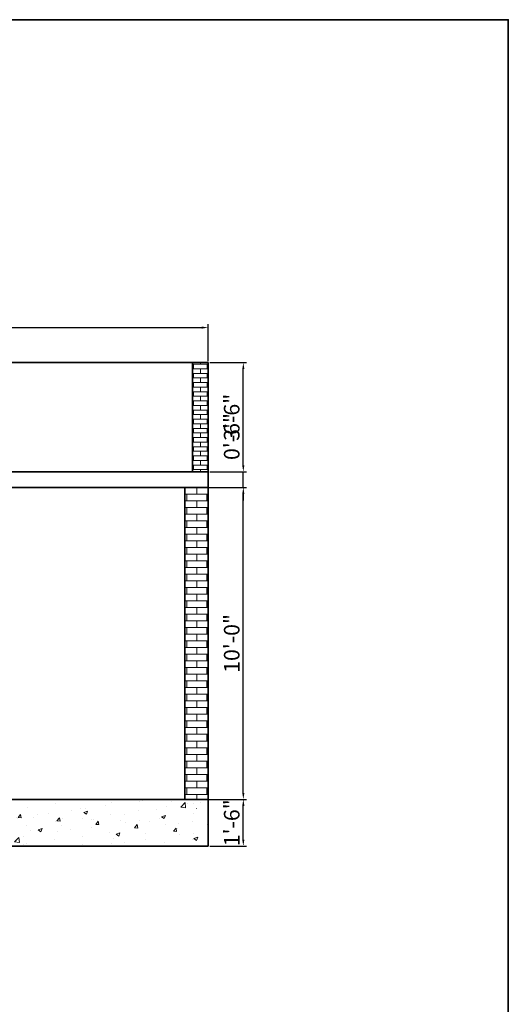
# Model space of a CAD drawing. Units: inches. Extents: x 2656 to 9931, y 1941 to 3068.
# Tile 46 of 46: x 3328 to 3515, y 2689 to 3068. Entities that reach past the tile are written whole.
import ezdxf

# ---------------------------------------------------------------- set-up
doc = ezdxf.new("R2010")
doc.units = ezdxf.units.IN
for name, color, linetype, lineweight in [('A-ANNO-DIMS', 2, 'Continuous', 18), ('A-ANNO-TTLB', 7, 'Continuous', 35), ('A-SECT', 7, 'Continuous', 35), ('A-SECT-PATT', 251, 'Continuous', 13), ('S-FNDN-PATT', 8, 'Continuous', 13)]:
    doc.layers.add(name, color=color, linetype=linetype, lineweight=lineweight)
doc.styles.get("Standard").update_dxf_attribs({"font": 'arial.ttf'})
doc.dimstyles.new('ISO-25', dxfattribs={"dimtxt": 6, "dimasz": 2.5, "dimexe": 1.25, "dimexo": 0.625, "dimtad": 1, "dimdec": 0, "dimlunit": 3, "dimtxsty": 'Standard', "dimcen": 2.5, "dimadec": 0, "dimazin": 0, "dimtfac": 1, "dimtdec": 0, "dimtmove": 0, "dimatfit": 3, "dimfxl": 1, "dimarcsym": 0})

# ---------------------------------------------------------------- blocks, each defined once
blk = doc.blocks.new('*D89')
at = {"layer": 'A-ANNO-DIMS', "color": 0, "lineweight": -2, "transparency": 16777216}
for p, q in [((3145.05, 2936.52), (3145.05, 2950.64)), ((3147.55, 2949.39), (3397.55, 2949.39)), ((3400.05, 2936.52), (3400.05, 2950.64))]:
    blk.add_line(p, q, dxfattribs=at)
at = {"layer": 'A-ANNO-DIMS', "color": 0, "transparency": 16777216}
for points in [[(3147.55, 2949.81), (3147.55, 2948.98), (3145.05, 2949.39)], [(3397.55, 2949.81), (3397.55, 2948.98), (3400.05, 2949.39)]]:
    blk.add_solid(points, dxfattribs=at)
at = {"layer": 'Defpoints', "color": 0, "transparency": 16777216}
for p in [(3400.05, 2949.39), (3145.05, 2935.89), (3400.05, 2935.89)]:
    blk.add_point(p, dxfattribs=at)
at = {"layer": 'A-ANNO-DIMS', "color": 0, "transparency": 16777216, "insert": (3272.55, 2953.08), "char_height": 6, "attachment_point": 5}
blk.add_mtext('21\'-3"', dxfattribs=at)
blk = doc.blocks.new('*D91')
at = {"layer": 'A-ANNO-DIMS', "color": 0, "lineweight": -2, "transparency": 16777216}
for p, q in [((3400.67, 2767.89), (3414.8, 2767.89)), ((3413.55, 2752.39), (3413.55, 2765.39)), ((3400.67, 2749.89), (3414.8, 2749.89))]:
    blk.add_line(p, q, dxfattribs=at)
at = {"layer": 'A-ANNO-DIMS', "color": 0, "transparency": 16777216}
for points in [[(3413.13, 2765.39), (3413.96, 2765.39), (3413.55, 2767.89)], [(3413.13, 2752.39), (3413.96, 2752.39), (3413.55, 2749.89)]]:
    blk.add_solid(points, dxfattribs=at)
at = {"layer": 'Defpoints', "color": 0, "transparency": 16777216}
for p in [(3400.05, 2767.89), (3413.55, 2767.89), (3400.05, 2749.89)]:
    blk.add_point(p, dxfattribs=at)
at = {"layer": 'A-ANNO-DIMS', "color": 0, "transparency": 16777216, "insert": (3409.86, 2758.89), "char_height": 6, "attachment_point": 5, "rotation": 90}
blk.add_mtext('1\'-6"', dxfattribs=at)
blk = doc.blocks.new('*D92')
at = {"layer": 'A-ANNO-DIMS', "color": 0, "lineweight": -2, "transparency": 16777216}
for p, q in [((3391.67, 2887.89), (3414.8, 2887.89)), ((3413.55, 2770.39), (3413.55, 2885.39)), ((3391.67, 2767.89), (3414.8, 2767.89))]:
    blk.add_line(p, q, dxfattribs=at)
at = {"layer": 'A-ANNO-DIMS', "color": 0, "transparency": 16777216}
for points in [[(3413.13, 2885.39), (3413.96, 2885.39), (3413.55, 2887.89)], [(3413.13, 2770.39), (3413.96, 2770.39), (3413.55, 2767.89)]]:
    blk.add_solid(points, dxfattribs=at)
at = {"layer": 'Defpoints', "color": 0, "transparency": 16777216}
for p in [(3391.05, 2887.89), (3413.55, 2887.89), (3391.05, 2767.89)]:
    blk.add_point(p, dxfattribs=at)
at = {"layer": 'A-ANNO-DIMS', "color": 0, "transparency": 16777216, "insert": (3409.86, 2827.89), "char_height": 6, "attachment_point": 5, "rotation": 90}
blk.add_mtext('10\'-0"', dxfattribs=at)
blk = doc.blocks.new('*D93')
at = {"layer": 'A-ANNO-DIMS', "color": 0, "lineweight": -2, "transparency": 16777216}
for p, q in [((3413.55, 2896.39), (3413.55, 2916.09)), ((3400.67, 2893.89), (3414.8, 2893.89)), ((3413.55, 2887.89), (3413.55, 2893.89)), ((3400.67, 2887.89), (3414.8, 2887.89)), ((3413.55, 2885.39), (3413.55, 2882.89))]:
    blk.add_line(p, q, dxfattribs=at)
at = {"layer": 'A-ANNO-DIMS', "color": 0, "transparency": 16777216}
for points in [[(3413.13, 2896.39), (3413.96, 2896.39), (3413.55, 2893.89)], [(3413.13, 2885.39), (3413.96, 2885.39), (3413.55, 2887.89)]]:
    blk.add_solid(points, dxfattribs=at)
at = {"layer": 'Defpoints', "color": 0, "transparency": 16777216}
for p in [(3400.05, 2893.89), (3413.55, 2893.89), (3400.05, 2887.89)]:
    blk.add_point(p, dxfattribs=at)
at = {"layer": 'A-ANNO-DIMS', "color": 0, "transparency": 16777216, "insert": (3409.86, 2907.49), "char_height": 6, "attachment_point": 5, "rotation": 90}
blk.add_mtext('0\'-6"', dxfattribs=at)
blk = doc.blocks.new('*D94')
at = {"layer": 'A-ANNO-DIMS', "color": 0, "lineweight": -2, "transparency": 16777216}
for p, q in [((3400.67, 2935.89), (3414.8, 2935.89)), ((3413.55, 2896.39), (3413.55, 2933.39)), ((3400.67, 2893.89), (3414.8, 2893.89))]:
    blk.add_line(p, q, dxfattribs=at)
at = {"layer": 'A-ANNO-DIMS', "color": 0, "transparency": 16777216}
for points in [[(3413.13, 2933.39), (3413.96, 2933.39), (3413.55, 2935.89)], [(3413.13, 2896.39), (3413.96, 2896.39), (3413.55, 2893.89)]]:
    blk.add_solid(points, dxfattribs=at)
at = {"layer": 'Defpoints', "color": 0, "transparency": 16777216}
for p in [(3400.05, 2935.89), (3413.55, 2935.89), (3400.05, 2893.89)]:
    blk.add_point(p, dxfattribs=at)
at = {"layer": 'A-ANNO-DIMS', "color": 0, "transparency": 16777216, "insert": (3409.85, 2914.89), "char_height": 6, "attachment_point": 5, "rotation": 90}
blk.add_mtext('3\'-6"', dxfattribs=at)

msp = doc.modelspace()

# ---------------------------------------------------------------- hatches: boundary and pattern name
at = {"layer": 'A-SECT-PATT'}
h = msp.add_hatch(dxfattribs=at)
h.set_pattern_fill('AR-SAND', color=256, scale=2)
h.set_pattern_definition([(37.5, (0, 64.96), (-3.2, 97.8826), [0, -77.216, 0, -86.36, 0, -82.55]), (7.5, (0, 64.96), (89.9047, 143.365), [0, -41.656, 0, -69.596, 0, -26.67]), (327.5, (-62.48, 64.96), (158.1985, 0.2874), [0, -25.4, 0, -91.44, 0, -119.38]), (317.5, (-62.48, 64.96), (152.7113, 44.586), [0, -12.7, 0, -59.944, 0, -68.58])])
h.paths.add_polyline_path([(3394.03, 2893.89), (3394.03, 2935.89), (3150.15, 2935.89), (3150.15, 2893.89)])
h = msp.add_hatch(dxfattribs=at)
h.set_pattern_fill('AR-BRSTD', color=256, scale=0.02604005, style=0)
h.paths.add_polyline_path([(3394.03, 2893.89), (3400.05, 2893.89), (3400.05, 2935.89), (3394.03, 2935.89)])
h = msp.add_hatch(dxfattribs=at)
h.set_pattern_fill('AR-BRSTD', color=256, scale=0.0378939, style=0)
h.paths.add_polyline_path([(3391.05, 2767.89), (3400.05, 2767.89), (3400.05, 2887.89), (3391.05, 2887.89)])
at = {"layer": 'S-FNDN-PATT'}
h = msp.add_hatch(dxfattribs=at)
h.set_pattern_fill('AR-CONC', color=256, scale=0.082, style=0)
h.paths.add_polyline_path([(3145.05, 2749.89), (3400.05, 2749.89), (3400.05, 2767.89), (3145.05, 2767.89)])

# ---------------------------------------------------------------- linework, layer by layer
at = {"layer": 'A-ANNO-TTLB'}
msp.add_lwpolyline([(2655.77, 3067.84), (3515.43, 3067.84), (3515.43, 1940.89), (2655.77, 1940.89)], close=True, dxfattribs=at)
at = {"layer": 'A-SECT'}
for p, q in [((3145.05, 2935.89), (3400.05, 2935.89)), ((3394.03, 2893.89), (3394.03, 2935.89)), ((3400.05, 2935.89), (3400.05, 2749.89)), ((3400.05, 2935.89), (3400.05, 2749.89)), ((3145.05, 2893.89), (3400.05, 2893.89)), ((3145.05, 2887.89), (3400.05, 2887.89)), ((3391.05, 2887.89), (3391.05, 2767.89)), ((3145.05, 2767.89), (3400.05, 2767.89)), ((3145.05, 2749.89), (3400.05, 2749.89)), ((3145.05, 2749.89), (3400.05, 2749.89))]:
    msp.add_line(p, q, dxfattribs=at)
at = {"layer": 'A-SECT-PATT'}
msp.add_line((3395.55, 2764.41), (3395.55, 2764.49), dxfattribs=at)

# ---------------------------------------------------------------- dimensions: what is measured, and where the dimension line sits
at = {"layer": 'A-ANNO-DIMS'}
dim = msp.add_linear_dim(base=(3400.05, 2949.39), p1=(3145.05, 2935.89), p2=(3400.05, 2935.89), dimstyle='ISO-25', override={"dimdec": 1, "dimlfac": 1, "dimrnd": 0, "dimzin": 1, "dimdsep": 46, "dimlunit": 4, "dimfrac": 2}, dxfattribs=at)
dim.commit()
dim.dimension.update_dxf_attribs({"geometry": '*D89', "text_midpoint": (3272.55, 2953.08)})
for base, p1, p2, picture, middle in [((3413.55, 2935.89), (3400.05, 2893.89), (3400.05, 2935.89), '*D94', (3409.85, 2914.89)), ((3413.55, 2893.89), (3400.05, 2887.89), (3400.05, 2893.89), '*D93', (3409.86, 2907.49)), ((3413.55, 2887.89), (3391.05, 2767.89), (3391.05, 2887.89), '*D92', (3409.86, 2827.89)), ((3413.55, 2767.89), (3400.05, 2749.89), (3400.05, 2767.89), '*D91', (3409.86, 2758.89))]:
    dim = msp.add_linear_dim(base=base, p1=p1, p2=p2, angle=90, dimstyle='ISO-25', override={"dimdec": 1, "dimlfac": 1, "dimrnd": 0, "dimzin": 1, "dimdsep": 46, "dimlunit": 4, "dimfrac": 2}, dxfattribs=at)
    dim.commit()
    dim.dimension.update_dxf_attribs({"geometry": picture, "text_midpoint": middle})

doc.saveas('drawing.dxf')
